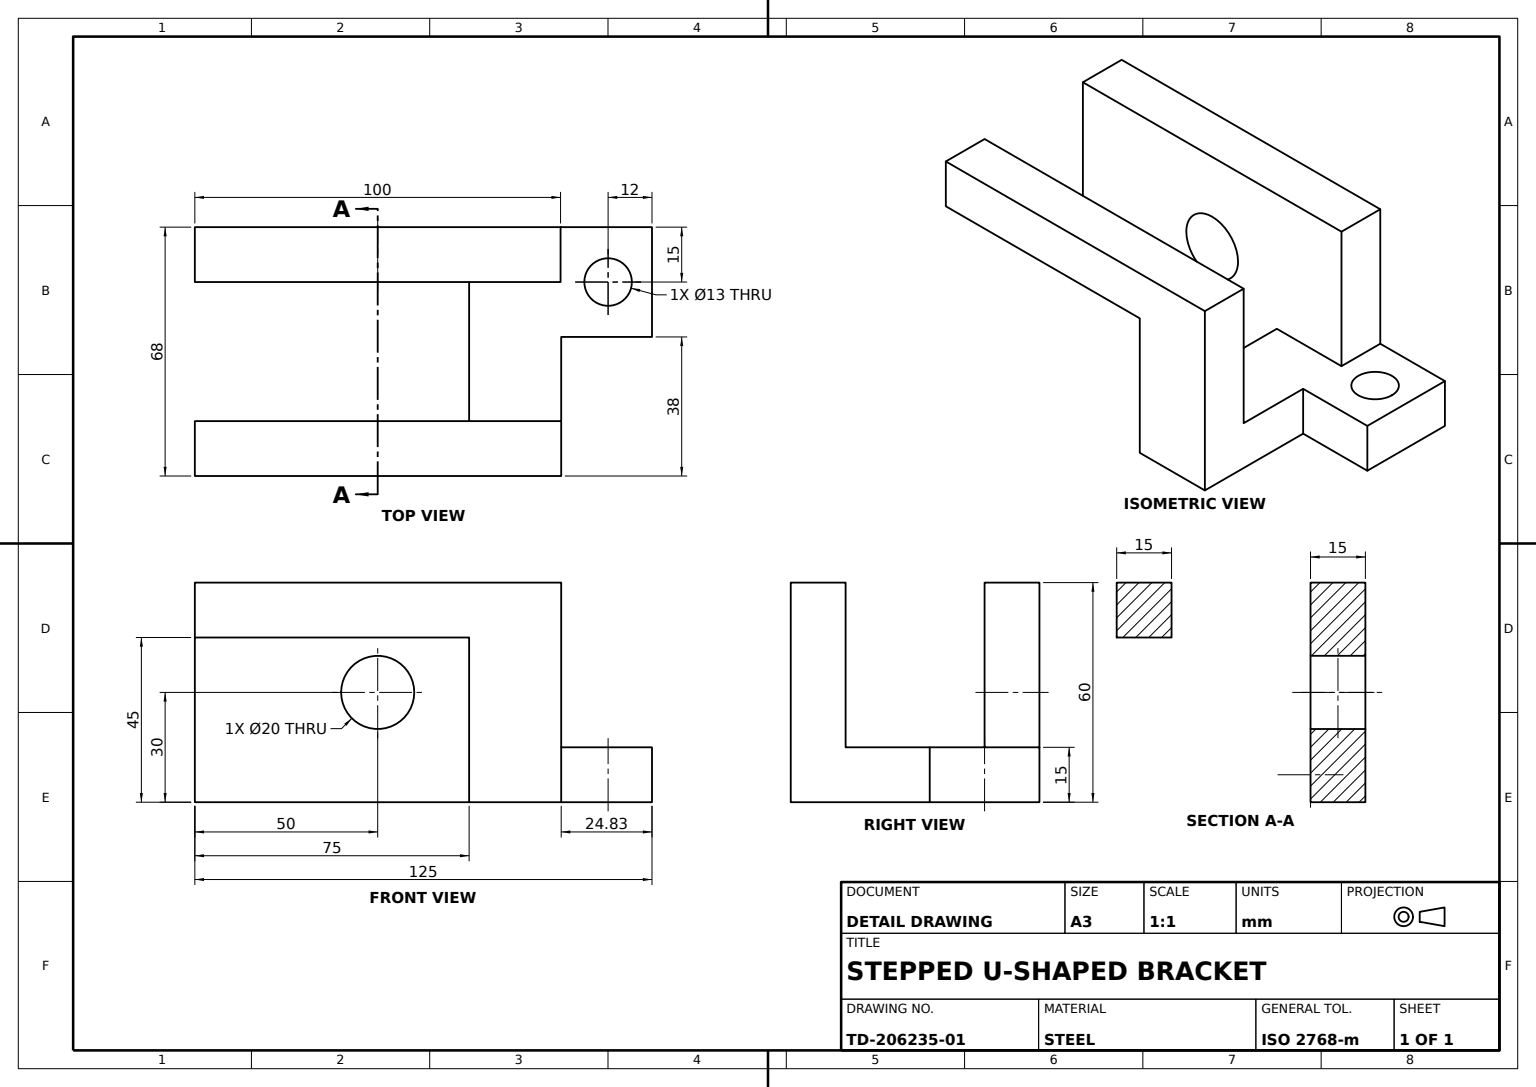
from build123d import *

# Parameters (mm, degrees)
BASE_PLATE_SKETCH_W     = 100
BASE_PLATE_SKETCH_H     = 60
BASE_PLATE_DEPTH        = 15
UPRIGHT_BLOCK_SKETCH_W  = 50
UPRIGHT_BLOCK_SKETCH_H  = 15
UPRIGHT_BLOCK_DEPTH     = 30
SIDE_WALL_SKETCH_W      = 25.174411278
SIDE_WALL_SKETCH_H      = 15
SIDE_WALL_DEPTH         = 38
LOWER_ARM_SKETCH_W      = 25.174411278
LOWER_ARM_SKETCH_H      = 15
LOWER_ARM_DEPTH         = 45
UPPER_ARM_SKETCH_W      = 15
UPPER_ARM_SKETCH_H      = 15
UPPER_ARM_DEPTH         = 75
WALL_HOLE_SKETCH_R      = 6.5
WALL_THROUGH_HOLE_DEPTH = 75
BASE_HOLE_SKETCH_R      = 10
BASE_THROUGH_HOLE_DEPTH = 75


with BuildPart() as part:
    # Base Plate Sketch → Base Plate (new body)
    with BuildSketch(Plane.XY):
        Rectangle(BASE_PLATE_SKETCH_W, BASE_PLATE_SKETCH_H)
    extrude(amount=BASE_PLATE_DEPTH)

    # Upright Block Sketch → Upright Block (add)
    with BuildSketch(Plane(origin=(0, 0, 0), x_dir=(-1, 0, 0), z_dir=(0, 0, -1))):
        with Locations((-50, -22.5)):
            Rectangle(UPRIGHT_BLOCK_SKETCH_W, UPRIGHT_BLOCK_SKETCH_H)
    extrude(amount=-UPRIGHT_BLOCK_DEPTH)

    # Side Wall Sketch → Side Wall (add)
    with BuildSketch(Plane.XY.offset(30)):
        with Locations((37.587205639, -22.5)):
            Rectangle(SIDE_WALL_SKETCH_W, SIDE_WALL_SKETCH_H)
    extrude(amount=SIDE_WALL_DEPTH)

    # Lower Arm Sketch → Lower Arm (add)
    with BuildSketch(Plane(origin=(0, -15, 0), x_dir=(1, 0, 0), z_dir=(0, 1, 0))):
        with Locations((37.587205639, -60.5)):
            Rectangle(LOWER_ARM_SKETCH_W, LOWER_ARM_SKETCH_H)
    extrude(amount=LOWER_ARM_DEPTH)

    # Upper Arm Sketch → Upper Arm (add)
    with BuildSketch(Plane.ZY.offset(-25)):
        with Locations((60.5, 22.5)):
            Rectangle(UPPER_ARM_SKETCH_W, UPPER_ARM_SKETCH_H)
    extrude(amount=UPPER_ARM_DEPTH)

    # Wall Hole Sketch → Wall Through Hole (cut)
    with BuildSketch(Plane(origin=(0, -15, 0), x_dir=(1, 0, 0), z_dir=(0, 1, 0))):
        with Locations(Location((63, -15, 0), (0, 0, 180))):
            Circle(WALL_HOLE_SKETCH_R)
    extrude(amount=-WALL_THROUGH_HOLE_DEPTH, mode=Mode.SUBTRACT)

    # Base Hole Sketch → Base Through Hole (cut)
    with BuildSketch(Plane.XY.offset(15)):
        Circle(BASE_HOLE_SKETCH_R)
    extrude(amount=-BASE_THROUGH_HOLE_DEPTH, mode=Mode.SUBTRACT)


solid = part.part
